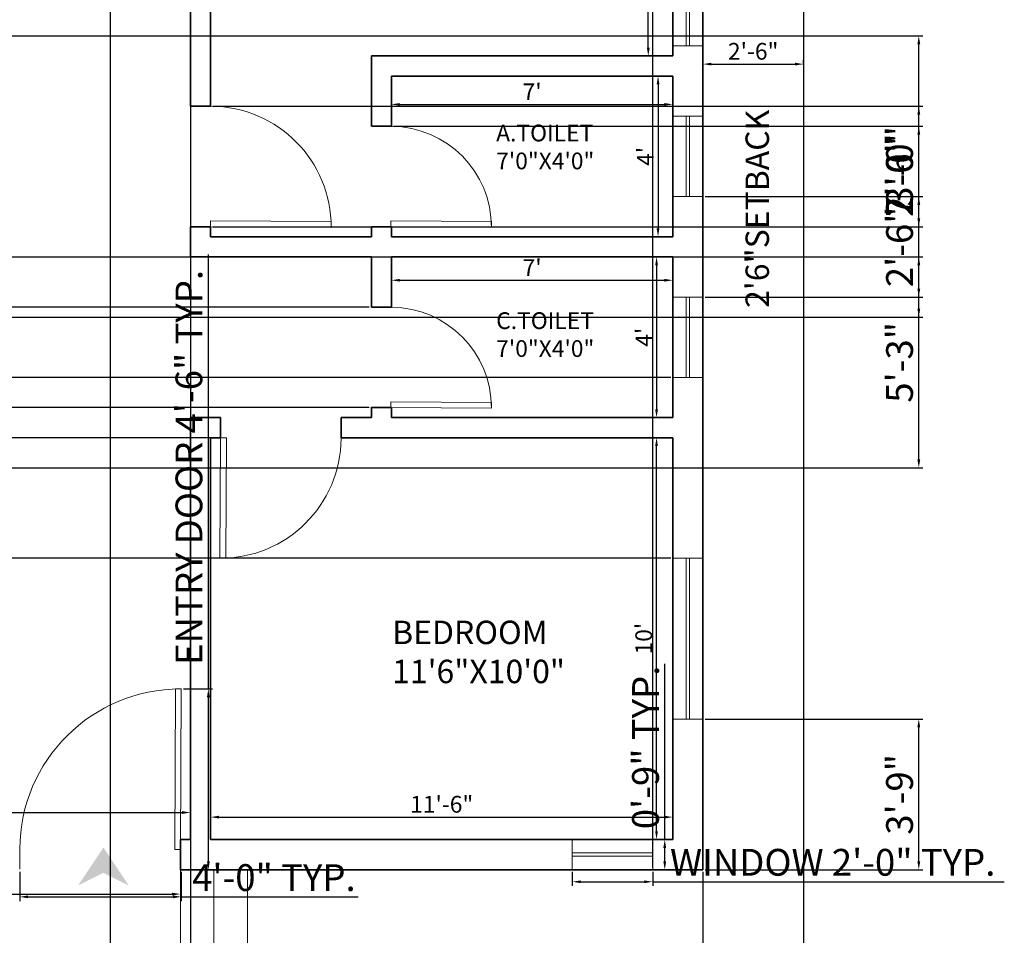
# Model space of a CAD drawing. Units: inches. Extents: x 3394 to 4794, y 965 to 1718.
# Tile 14 of 15: x 4500 to 4794, y 1179 to 1453. Entities that reach past the tile are written whole.
import ezdxf

# ---------------------------------------------------------------- set-up
doc = ezdxf.new("R2010")
doc.units = ezdxf.units.IN
for name, color, linetype, lineweight in [('A-ANNO-DIMS', 2, 'Continuous', 13), ('A-ANNO-PATT', 1, 'Continuous', 13), ('A-ANNO-TEXT', 7, 'Continuous', 18), ('A-AREA-IDEN', 7, 'Continuous', 18), ('A-DOOR', 4, 'Continuous', 18), ('A-FLOR-STRS', 7, 'Continuous', 18), ('A-GLAZ', 4, 'Continuous', 18), ('A-WALL', 7, 'Continuous', 35), ('C-PROP', 7, 'Continuous', 25)]:
    doc.layers.add(name, color=color, linetype=linetype, lineweight=lineweight)
doc.styles.get("Standard").update_dxf_attribs({"font": 'arial.ttf'})
doc.dimstyles.new('ISO-25', dxfattribs={"dimtxt": 8, "dimasz": 2.5, "dimexe": 1.25, "dimexo": 0.625, "dimtad": 1, "dimlunit": 3, "dimtxsty": 'Standard', "dimcen": 2.5, "dimadec": 0, "dimazin": 0, "dimtfac": 1, "dimtmove": 0, "dimatfit": 3, "dimfxl": 1, "dimarcsym": 0})

# ---------------------------------------------------------------- blocks, each defined once
blk = doc.blocks.new('*U5')
for p, q in [((0, 0), (0, -6)), ((30, 0), (30, -6))]:
    blk.add_line(p, q)
blk.add_lwpolyline([(0, 0), (0, 30), (1.75, 30), (1.75, 0)], close=True)
blk.add_arc((0, 0), 30, 0, 90)
blk = doc.blocks.new('*U11')
for p, q in [((0, 0), (0, -6)), ((36, 0), (36, -6))]:
    blk.add_line(p, q)
blk.add_lwpolyline([(0, 0), (0, 36), (1.75, 36), (1.75, 0)], close=True)
blk.add_arc((0, 0), 36, 0, 90)
blk = doc.blocks.new('*D36')
at = {"layer": 'A-ANNO-DIMS', "color": 0, "lineweight": -2, "transparency": 16777216}
for p, q in [((4419.27, 1198.06), (4419.27, 1190.15)), ((4548.27, 1198.06), (4548.27, 1190.15)), ((4421.77, 1191.4), (4545.77, 1191.4))]:
    blk.add_line(p, q, dxfattribs=at)
at = {"layer": 'A-ANNO-DIMS', "color": 0, "transparency": 16777216}
for points in [[(4421.77, 1191.81), (4421.77, 1190.98), (4419.27, 1191.4)], [(4545.77, 1191.81), (4545.77, 1190.98), (4548.27, 1191.4)]]:
    blk.add_solid(points, dxfattribs=at)
at = {"layer": 'Defpoints', "color": 0, "transparency": 16777216}
for p in [(4419.27, 1198.68), (4548.27, 1198.68), (4548.27, 1191.4)]:
    blk.add_point(p, dxfattribs=at)
at = {"layer": 'A-ANNO-DIMS', "color": 0, "transparency": 16777216, "insert": (4483.77, 1194.58), "char_height": 5, "attachment_point": 5}
blk.add_mtext('10\'-9"', dxfattribs=at)
blk = doc.blocks.new('*D38')
at = {"layer": 'A-ANNO-DIMS', "color": 0, "lineweight": -2, "transparency": 16777216}
for p, q in [((4704.27, 1439.09), (4704.27, 1440.48)), ((4706.77, 1439.23), (4731.77, 1439.23)), ((4734.27, 1439.09), (4734.27, 1440.48))]:
    blk.add_line(p, q, dxfattribs=at)
at = {"layer": 'A-ANNO-DIMS', "color": 0, "transparency": 16777216}
for points in [[(4706.77, 1439.65), (4706.77, 1438.82), (4704.27, 1439.23)], [(4731.77, 1439.65), (4731.77, 1438.82), (4734.27, 1439.23)]]:
    blk.add_solid(points, dxfattribs=at)
at = {"layer": 'Defpoints', "color": 0, "transparency": 16777216}
for p in [(4704.27, 1438.47), (4734.27, 1439.23), (4734.27, 1438.47)]:
    blk.add_point(p, dxfattribs=at)
at = {"layer": 'A-ANNO-DIMS', "color": 0, "transparency": 16777216, "insert": (4719.27, 1442.41), "char_height": 5, "attachment_point": 5}
blk.add_mtext('2\'-6"', dxfattribs=at)
blk = doc.blocks.new('*D41')
at = {"layer": 'A-ANNO-DIMS', "color": 0, "lineweight": -2, "transparency": 16777216}
for p, q in [((4350.27, 1208.31), (4350.27, 1217.01)), ((4352.77, 1215.76), (4548.77, 1215.76)), ((4551.27, 1208.31), (4551.27, 1217.01))]:
    blk.add_line(p, q, dxfattribs=at)
at = {"layer": 'A-ANNO-DIMS', "color": 0, "transparency": 16777216}
for points in [[(4352.77, 1216.17), (4352.77, 1215.34), (4350.27, 1215.76)], [(4548.77, 1216.17), (4548.77, 1215.34), (4551.27, 1215.76)]]:
    blk.add_solid(points, dxfattribs=at)
at = {"layer": 'Defpoints', "color": 0, "transparency": 16777216}
for p in [(4551.27, 1215.76), (4350.27, 1207.68), (4551.27, 1207.68)]:
    blk.add_point(p, dxfattribs=at)
at = {"layer": 'A-ANNO-DIMS', "color": 0, "transparency": 16777216, "insert": (4450.77, 1218.94), "char_height": 5, "attachment_point": 5}
blk.add_mtext('16\'-9"', dxfattribs=at)
blk = doc.blocks.new('*D42')
at = {"layer": 'A-ANNO-DIMS', "color": 0, "lineweight": -2, "transparency": 16777216}
for p, q in [((4557.27, 1208.31), (4557.27, 1215.64)), ((4559.77, 1214.39), (4692.77, 1214.39)), ((4695.27, 1208.31), (4695.27, 1215.64))]:
    blk.add_line(p, q, dxfattribs=at)
at = {"layer": 'A-ANNO-DIMS', "color": 0, "transparency": 16777216}
for points in [[(4559.77, 1214.8), (4559.77, 1213.97), (4557.27, 1214.39)], [(4692.77, 1214.8), (4692.77, 1213.97), (4695.27, 1214.39)]]:
    blk.add_solid(points, dxfattribs=at)
at = {"layer": 'Defpoints', "color": 0, "transparency": 16777216}
for p in [(4695.27, 1214.39), (4557.27, 1207.68), (4695.27, 1207.68)]:
    blk.add_point(p, dxfattribs=at)
at = {"layer": 'A-ANNO-DIMS', "color": 0, "transparency": 16777216, "insert": (4626.27, 1217.57), "char_height": 5, "attachment_point": 5}
blk.add_mtext('11\'-6"', dxfattribs=at)
blk = doc.blocks.new('*D43')
at = {"layer": 'A-ANNO-DIMS', "color": 0, "lineweight": -2, "transparency": 16777216}
for p, q in [((4694.65, 1327.68), (4689.17, 1327.68)), ((4690.42, 1210.18), (4690.42, 1325.18)), ((4694.65, 1207.68), (4689.17, 1207.68))]:
    blk.add_line(p, q, dxfattribs=at)
at = {"layer": 'A-ANNO-DIMS', "color": 0, "transparency": 16777216}
for points in [[(4690, 1325.18), (4690.83, 1325.18), (4690.42, 1327.68)], [(4690, 1210.18), (4690.83, 1210.18), (4690.42, 1207.68)]]:
    blk.add_solid(points, dxfattribs=at)
at = {"layer": 'Defpoints', "color": 0, "transparency": 16777216}
for p in [(4690.42, 1327.68), (4695.27, 1327.68), (4695.27, 1207.68)]:
    blk.add_point(p, dxfattribs=at)
at = {"layer": 'A-ANNO-DIMS', "color": 0, "transparency": 16777216, "insert": (4687.24, 1267.68), "char_height": 5, "attachment_point": 5, "rotation": 90}
blk.add_mtext("10'", dxfattribs=at)
blk = doc.blocks.new('*D44')
at = {"layer": 'A-ANNO-DIMS', "color": 0, "lineweight": -2, "transparency": 16777216}
for p, q in [((4611.27, 1381.06), (4611.27, 1373.45)), ((4695.27, 1381.06), (4695.27, 1373.45)), ((4613.77, 1374.7), (4692.77, 1374.7))]:
    blk.add_line(p, q, dxfattribs=at)
at = {"layer": 'A-ANNO-DIMS', "color": 0, "transparency": 16777216}
for points in [[(4613.77, 1375.11), (4613.77, 1374.28), (4611.27, 1374.7)], [(4692.77, 1375.11), (4692.77, 1374.28), (4695.27, 1374.7)]]:
    blk.add_solid(points, dxfattribs=at)
at = {"layer": 'Defpoints', "color": 0, "transparency": 16777216}
for p in [(4611.27, 1381.68), (4695.27, 1381.68), (4695.27, 1374.7)]:
    blk.add_point(p, dxfattribs=at)
at = {"layer": 'A-ANNO-DIMS', "color": 0, "transparency": 16777216, "insert": (4653.27, 1377.82), "char_height": 5, "attachment_point": 5}
blk.add_mtext("7'", dxfattribs=at)
blk = doc.blocks.new('*D45')
at = {"layer": 'A-ANNO-DIMS', "color": 0, "lineweight": -2, "transparency": 16777216}
for p, q in [((4694.65, 1381.68), (4689.18, 1381.68)), ((4690.43, 1379.18), (4690.43, 1336.18)), ((4694.65, 1333.68), (4689.18, 1333.68))]:
    blk.add_line(p, q, dxfattribs=at)
at = {"layer": 'A-ANNO-DIMS', "color": 0, "transparency": 16777216}
for points in [[(4690.01, 1379.18), (4690.84, 1379.18), (4690.43, 1381.68)], [(4690.01, 1336.18), (4690.84, 1336.18), (4690.43, 1333.68)]]:
    blk.add_solid(points, dxfattribs=at)
at = {"layer": 'Defpoints', "color": 0, "transparency": 16777216}
for p in [(4695.27, 1381.68), (4690.43, 1333.68), (4695.27, 1333.68)]:
    blk.add_point(p, dxfattribs=at)
at = {"layer": 'A-ANNO-DIMS', "color": 0, "transparency": 16777216, "insert": (4687.3, 1357.68), "char_height": 5, "attachment_point": 5, "rotation": 90}
blk.add_mtext("4'", dxfattribs=at)
blk = doc.blocks.new('*D46')
at = {"layer": 'A-ANNO-DIMS', "color": 0, "lineweight": -2, "transparency": 16777216}
for p, q in [((4694.65, 1435.68), (4689.62, 1435.68)), ((4690.87, 1433.18), (4690.87, 1390.18)), ((4694.65, 1387.68), (4689.62, 1387.68))]:
    blk.add_line(p, q, dxfattribs=at)
at = {"layer": 'A-ANNO-DIMS', "color": 0, "transparency": 16777216}
for points in [[(4690.45, 1433.18), (4691.28, 1433.18), (4690.87, 1435.68)], [(4690.45, 1390.18), (4691.28, 1390.18), (4690.87, 1387.68)]]:
    blk.add_solid(points, dxfattribs=at)
at = {"layer": 'Defpoints', "color": 0, "transparency": 16777216}
for p in [(4695.27, 1435.68), (4690.87, 1387.68), (4695.27, 1387.68)]:
    blk.add_point(p, dxfattribs=at)
at = {"layer": 'A-ANNO-DIMS', "color": 0, "transparency": 16777216, "insert": (4687.74, 1411.68), "char_height": 5, "attachment_point": 5, "rotation": 90}
blk.add_mtext("4'", dxfattribs=at)
blk = doc.blocks.new('*D47')
at = {"layer": 'A-ANNO-DIMS', "color": 0, "lineweight": -2, "transparency": 16777216}
for p, q in [((4611.27, 1435.06), (4611.27, 1425.96)), ((4695.27, 1435.06), (4695.27, 1425.96)), ((4613.77, 1427.21), (4692.77, 1427.21))]:
    blk.add_line(p, q, dxfattribs=at)
at = {"layer": 'A-ANNO-DIMS', "color": 0, "transparency": 16777216}
for points in [[(4613.77, 1427.62), (4613.77, 1426.79), (4611.27, 1427.21)], [(4692.77, 1427.62), (4692.77, 1426.79), (4695.27, 1427.21)]]:
    blk.add_solid(points, dxfattribs=at)
at = {"layer": 'Defpoints', "color": 0, "transparency": 16777216}
for p in [(4611.27, 1435.68), (4695.27, 1435.68), (4695.27, 1427.21)]:
    blk.add_point(p, dxfattribs=at)
at = {"layer": 'A-ANNO-DIMS', "color": 0, "transparency": 16777216, "insert": (4653.27, 1430.33), "char_height": 5, "attachment_point": 5}
blk.add_mtext("7'", dxfattribs=at)
blk = doc.blocks.new('*D48')
at = {"layer": 'A-ANNO-DIMS', "color": 0, "lineweight": -2, "transparency": 16777216}
for p, q in [((4694.65, 1573.68), (4686.7, 1573.68)), ((4687.95, 1444.18), (4687.95, 1571.18)), ((4694.65, 1441.68), (4686.7, 1441.68))]:
    blk.add_line(p, q, dxfattribs=at)
at = {"layer": 'A-ANNO-DIMS', "color": 0, "transparency": 16777216}
for points in [[(4687.53, 1571.18), (4688.37, 1571.18), (4687.95, 1573.68)], [(4687.53, 1444.18), (4688.37, 1444.18), (4687.95, 1441.68)]]:
    blk.add_solid(points, dxfattribs=at)
at = {"layer": 'Defpoints', "color": 0, "transparency": 16777216}
for p in [(4687.95, 1573.68), (4695.27, 1573.68), (4695.27, 1441.68)]:
    blk.add_point(p, dxfattribs=at)
at = {"layer": 'A-ANNO-DIMS', "color": 0, "transparency": 16777216, "insert": (4684.81, 1507.68), "char_height": 5, "attachment_point": 5, "rotation": 90}
blk.add_mtext("11'", dxfattribs=at)
blk = doc.blocks.new('WIN-48IN')
for p, q in [((9, 48), (0, 48)), ((4, 0), (4, 48)), ((5, 0), (5, 48)), ((9, 0), (0, 0))]:
    blk.add_line(p, q)
blk = doc.blocks.new('WIN-24IN')
for p, q in [((0, 9), (0, 0)), ((24, 9), (24, 0)), ((0, 5), (24, 5)), ((0, 4), (24, 4))]:
    blk.add_line(p, q)
blk = doc.blocks.new('DOOR-ENTRY-48IN')
for p, q in [((0.03, 6.2), (0, 0.2)), ((48.03, 6), (48, 0))]:
    blk.add_line(p, q)
blk.add_lwpolyline([(48.03, 6), (48.24, 54), (46.49, 54.01), (46.28, 6.01)], close=True)
blk.add_arc((48.03, 6), 48, 90, 179.759)
blk = doc.blocks.new('STAIR-SITOUT-3STEP')
for p, q in [((129, 68), (129, 20)), ((139, 68), (139, 10)), ((149, 68), (149, 0)), ((0, 20), (129, 20)), ((0, 10), (139, 10)), ((0, 0), (149, 0))]:
    blk.add_line(p, q)
blk = doc.blocks.new('*D64')
at = {"layer": 'A-ANNO-DIMS', "color": 0, "lineweight": -2, "transparency": 16777216}
for p, q in [((4665.27, 1198.06), (4665.27, 1193.83)), ((4689.27, 1198.06), (4689.27, 1193.83)), ((4667.77, 1195.08), (4686.77, 1195.08)), ((4689.27, 1195.08), (4794.25, 1195.08))]:
    blk.add_line(p, q, dxfattribs=at)
at = {"layer": 'A-ANNO-DIMS', "color": 0, "transparency": 16777216}
for points in [[(4667.77, 1195.5), (4667.77, 1194.67), (4665.27, 1195.08)], [(4686.77, 1195.5), (4686.77, 1194.67), (4689.27, 1195.08)]]:
    blk.add_solid(points, dxfattribs=at)
at = {"layer": 'Defpoints', "color": 0, "transparency": 16777216}
for p in [(4665.27, 1198.68), (4689.27, 1198.68), (4689.27, 1195.08)]:
    blk.add_point(p, dxfattribs=at)
at = {"layer": 'A-ANNO-DIMS', "color": 0, "transparency": 16777216, "insert": (4743.01, 1199.85), "char_height": 8, "attachment_point": 5}
blk.add_mtext('WINDOW 2\'-0" TYP.', dxfattribs=at)
blk = doc.blocks.new('*D65')
at = {"layer": 'A-ANNO-DIMS', "color": 0, "lineweight": -2, "transparency": 16777216}
for p, q in [((4692.87, 1207.68), (4692.87, 1260.2)), ((4689.9, 1207.68), (4694.12, 1207.68)), ((4692.87, 1201.18), (4692.87, 1205.18)), ((4689.9, 1198.68), (4694.12, 1198.68))]:
    blk.add_line(p, q, dxfattribs=at)
at = {"layer": 'A-ANNO-DIMS', "color": 0, "transparency": 16777216}
for points in [[(4692.45, 1205.18), (4693.29, 1205.18), (4692.87, 1207.68)], [(4692.45, 1201.18), (4693.29, 1201.18), (4692.87, 1198.68)]]:
    blk.add_solid(points, dxfattribs=at)
at = {"layer": 'Defpoints', "color": 0, "transparency": 16777216}
for p in [(4689.27, 1207.68), (4692.87, 1207.68), (4689.27, 1198.68)]:
    blk.add_point(p, dxfattribs=at)
at = {"layer": 'A-ANNO-DIMS', "color": 0, "transparency": 16777216, "insert": (4688.16, 1235.19), "char_height": 8, "attachment_point": 5, "rotation": 90}
blk.add_mtext('0\'-9" TYP.', dxfattribs=at)
blk = doc.blocks.new('*D68')
at = {"layer": 'A-ANNO-DIMS', "color": 0, "lineweight": -2, "transparency": 16777216}
for p, q in [((4556.61, 1252.69), (4556.61, 1382.4)), ((4549.13, 1252.69), (4557.86, 1252.69)), ((4556.61, 1201.18), (4556.61, 1250.19)), ((4549.13, 1198.68), (4557.86, 1198.68))]:
    blk.add_line(p, q, dxfattribs=at)
at = {"layer": 'A-ANNO-DIMS', "color": 0, "transparency": 16777216}
for points in [[(4556.19, 1250.19), (4557.02, 1250.19), (4556.61, 1252.69)], [(4556.19, 1201.18), (4557.02, 1201.18), (4556.61, 1198.68)]]:
    blk.add_solid(points, dxfattribs=at)
at = {"layer": 'Defpoints', "color": 0, "transparency": 16777216}
for p in [(4548.51, 1252.69), (4556.61, 1252.69), (4548.51, 1198.68)]:
    blk.add_point(p, dxfattribs=at)
at = {"layer": 'A-ANNO-DIMS', "color": 0, "transparency": 16777216, "insert": (4551.84, 1318.8), "char_height": 8, "attachment_point": 5, "rotation": 90}
blk.add_mtext('ENTRY DOOR 4\'-6" TYP.', dxfattribs=at)
blk = doc.blocks.new('*D69')
at = {"layer": 'A-ANNO-DIMS', "color": 0, "lineweight": -2, "transparency": 16777216}
for p, q in [((4500.27, 1198.06), (4500.27, 1189.33)), ((4548.51, 1198.06), (4548.51, 1189.33)), ((4502.77, 1190.58), (4546.01, 1190.58)), ((4548.51, 1190.58), (4601.34, 1190.58))]:
    blk.add_line(p, q, dxfattribs=at)
at = {"layer": 'A-ANNO-DIMS', "color": 0, "transparency": 16777216}
for points in [[(4502.77, 1191), (4502.77, 1190.16), (4500.27, 1190.58)], [(4546.01, 1191), (4546.01, 1190.16), (4548.51, 1190.58)]]:
    blk.add_solid(points, dxfattribs=at)
at = {"layer": 'Defpoints', "color": 0, "transparency": 16777216}
for p in [(4500.27, 1198.68), (4548.51, 1198.68), (4548.51, 1190.58)]:
    blk.add_point(p, dxfattribs=at)
at = {"layer": 'A-ANNO-DIMS', "color": 0, "transparency": 16777216, "insert": (4576.17, 1195.29), "char_height": 8, "attachment_point": 5}
blk.add_mtext('4\'-0" TYP.', dxfattribs=at)
blk = doc.blocks.new('*D106')
at = {"layer": 'A-ANNO-DIMS', "color": 0, "lineweight": -2, "transparency": 16777216}
for p, q in [((4704.27, 1198.06), (4704.27, 987.36)), ((4341.27, 1117.06), (4341.27, 987.36)), ((4343.77, 988.61), (4701.77, 988.61))]:
    blk.add_line(p, q, dxfattribs=at)
at = {"layer": 'A-ANNO-DIMS', "color": 0, "transparency": 16777216}
for points in [[(4343.77, 989.03), (4343.77, 988.2), (4341.27, 988.61)], [(4701.77, 989.03), (4701.77, 988.2), (4704.27, 988.61)]]:
    blk.add_solid(points, dxfattribs=at)
at = {"layer": 'Defpoints', "color": 0, "transparency": 16777216}
for p in [(4704.27, 1198.68), (4341.27, 1117.68), (4704.27, 988.61)]:
    blk.add_point(p, dxfattribs=at)
at = {"layer": 'A-ANNO-DIMS', "color": 0, "transparency": 16777216, "insert": (4522.77, 993.32), "char_height": 8, "attachment_point": 5}
blk.add_mtext('30\'-3"', dxfattribs=at)
blk = doc.blocks.new('*D109')
at = {"layer": 'A-ANNO-DIMS', "color": 0, "lineweight": -2, "transparency": 16777216}
for p, q in [((4456.9, 1447.68), (4769.97, 1447.68)), ((4768.72, 1366.18), (4768.72, 1445.18)), ((4456.9, 1363.68), (4769.97, 1363.68))]:
    blk.add_line(p, q, dxfattribs=at)
at = {"layer": 'A-ANNO-DIMS', "color": 0, "transparency": 16777216}
for points in [[(4768.3, 1445.18), (4769.14, 1445.18), (4768.72, 1447.68)], [(4768.3, 1366.18), (4769.14, 1366.18), (4768.72, 1363.68)]]:
    blk.add_solid(points, dxfattribs=at)
at = {"layer": 'Defpoints', "color": 0, "transparency": 16777216}
for p in [(4456.27, 1447.68), (4768.72, 1447.68), (4456.27, 1363.68)]:
    blk.add_point(p, dxfattribs=at)
at = {"layer": 'A-ANNO-DIMS', "color": 0, "transparency": 16777216, "insert": (4764.01, 1405.68), "char_height": 8, "attachment_point": 5, "rotation": 90}
blk.add_mtext('7\'-0"', dxfattribs=at)
blk = doc.blocks.new('*D110')
at = {"layer": 'A-ANNO-DIMS', "color": 0, "lineweight": -2, "transparency": 16777216}
for p, q in [((4557.9, 1426.68), (4769.97, 1426.68)), ((4768.72, 1393.18), (4768.72, 1424.18)), ((4557.9, 1390.68), (4769.97, 1390.68))]:
    blk.add_line(p, q, dxfattribs=at)
at = {"layer": 'A-ANNO-DIMS', "color": 0, "transparency": 16777216}
for points in [[(4768.3, 1424.18), (4769.14, 1424.18), (4768.72, 1426.68)], [(4768.3, 1393.18), (4769.14, 1393.18), (4768.72, 1390.68)]]:
    blk.add_solid(points, dxfattribs=at)
at = {"layer": 'Defpoints', "color": 0, "transparency": 16777216}
for p in [(4557.27, 1426.68), (4768.72, 1426.68), (4557.27, 1390.68)]:
    blk.add_point(p, dxfattribs=at)
at = {"layer": 'A-ANNO-DIMS', "color": 0, "transparency": 16777216, "insert": (4764.01, 1408.68), "char_height": 8, "attachment_point": 5, "rotation": 90}
blk.add_mtext('3\'-0"', dxfattribs=at)
blk = doc.blocks.new('*D111')
at = {"layer": 'A-ANNO-DIMS', "color": 0, "lineweight": -2, "transparency": 16777216}
for p, q in [((4611.9, 1420.68), (4769.97, 1420.68)), ((4768.72, 1393.18), (4768.72, 1418.18)), ((4611.9, 1390.68), (4769.97, 1390.68))]:
    blk.add_line(p, q, dxfattribs=at)
at = {"layer": 'A-ANNO-DIMS', "color": 0, "transparency": 16777216}
for points in [[(4768.3, 1418.18), (4769.14, 1418.18), (4768.72, 1420.68)], [(4768.3, 1393.18), (4769.14, 1393.18), (4768.72, 1390.68)]]:
    blk.add_solid(points, dxfattribs=at)
at = {"layer": 'Defpoints', "color": 0, "transparency": 16777216}
for p in [(4611.27, 1420.68), (4768.72, 1420.68), (4611.27, 1390.68)]:
    blk.add_point(p, dxfattribs=at)
at = {"layer": 'A-ANNO-DIMS', "color": 0, "transparency": 16777216, "insert": (4764.01, 1405.68), "char_height": 8, "attachment_point": 5, "rotation": 90}
blk.add_mtext('2\'-6"', dxfattribs=at)
blk = doc.blocks.new('*D112')
at = {"layer": 'A-ANNO-DIMS', "color": 0, "lineweight": -2, "transparency": 16777216}
for p, q in [((4559.65, 1327.68), (4185.57, 1327.68)), ((4186.82, 1294.18), (4186.82, 1325.18)), ((4559.41, 1291.68), (4185.57, 1291.68))]:
    blk.add_line(p, q, dxfattribs=at)
at = {"layer": 'A-ANNO-DIMS', "color": 0, "transparency": 16777216}
for points in [[(4186.4, 1325.18), (4187.24, 1325.18), (4186.82, 1327.68)], [(4186.4, 1294.18), (4187.24, 1294.18), (4186.82, 1291.68)]]:
    blk.add_solid(points, dxfattribs=at)
at = {"layer": 'Defpoints', "color": 0, "transparency": 16777216}
for p in [(4186.82, 1327.68), (4560.27, 1327.68), (4560.03, 1291.68)]:
    blk.add_point(p, dxfattribs=at)
at = {"layer": 'A-ANNO-DIMS', "color": 0, "transparency": 16777216, "insert": (4182.11, 1309.68), "char_height": 8, "attachment_point": 5, "rotation": 90}
blk.add_mtext('3\'-0"', dxfattribs=at)
blk = doc.blocks.new('*D113')
at = {"layer": 'A-ANNO-DIMS', "color": 0, "lineweight": -2, "transparency": 16777216}
for p, q in [((4604.65, 1366.68), (4185.57, 1366.68)), ((4186.82, 1339.18), (4186.82, 1364.18)), ((4604.65, 1336.68), (4185.57, 1336.68))]:
    blk.add_line(p, q, dxfattribs=at)
at = {"layer": 'A-ANNO-DIMS', "color": 0, "transparency": 16777216}
for points in [[(4186.4, 1364.18), (4187.24, 1364.18), (4186.82, 1366.68)], [(4186.4, 1339.18), (4187.24, 1339.18), (4186.82, 1336.68)]]:
    blk.add_solid(points, dxfattribs=at)
at = {"layer": 'Defpoints', "color": 0, "transparency": 16777216}
for p in [(4186.82, 1366.68), (4605.27, 1366.68), (4605.27, 1336.68)]:
    blk.add_point(p, dxfattribs=at)
at = {"layer": 'A-ANNO-DIMS', "color": 0, "transparency": 16777216, "insert": (4182.11, 1351.68), "char_height": 8, "attachment_point": 5, "rotation": 90}
blk.add_mtext('2\'-6"', dxfattribs=at)
blk = doc.blocks.new('*D116')
at = {"layer": 'A-ANNO-DIMS', "color": 0, "lineweight": -2, "transparency": 16777216}
for p, q in [((4350.9, 1381.68), (4769.97, 1381.68)), ((4768.72, 1321.18), (4768.72, 1379.18)), ((4350.9, 1318.68), (4769.97, 1318.68))]:
    blk.add_line(p, q, dxfattribs=at)
at = {"layer": 'A-ANNO-DIMS', "color": 0, "transparency": 16777216}
for points in [[(4768.3, 1379.18), (4769.14, 1379.18), (4768.72, 1381.68)], [(4768.3, 1321.18), (4769.14, 1321.18), (4768.72, 1318.68)]]:
    blk.add_solid(points, dxfattribs=at)
at = {"layer": 'Defpoints', "color": 0, "transparency": 16777216}
for p in [(4350.27, 1381.68), (4768.72, 1381.68), (4350.27, 1318.68)]:
    blk.add_point(p, dxfattribs=at)
at = {"layer": 'A-ANNO-DIMS', "color": 0, "transparency": 16777216, "insert": (4764.01, 1350.18), "char_height": 8, "attachment_point": 5, "rotation": 90}
blk.add_mtext('5\'-3"', dxfattribs=at)
blk = doc.blocks.new('*D118')
at = {"layer": 'A-ANNO-DIMS', "color": 0, "lineweight": -2, "transparency": 16777216}
for p, q in [((4704.9, 1243.68), (4769.97, 1243.68)), ((4768.72, 1201.18), (4768.72, 1241.18)), ((4704.9, 1198.68), (4769.97, 1198.68))]:
    blk.add_line(p, q, dxfattribs=at)
at = {"layer": 'A-ANNO-DIMS', "color": 0, "transparency": 16777216}
for points in [[(4768.3, 1241.18), (4769.14, 1241.18), (4768.72, 1243.68)], [(4768.3, 1201.18), (4769.14, 1201.18), (4768.72, 1198.68)]]:
    blk.add_solid(points, dxfattribs=at)
at = {"layer": 'Defpoints', "color": 0, "transparency": 16777216}
for p in [(4704.27, 1243.68), (4768.72, 1243.68), (4704.27, 1198.68)]:
    blk.add_point(p, dxfattribs=at)
at = {"layer": 'A-ANNO-DIMS', "color": 0, "transparency": 16777216, "insert": (4764.01, 1221.18), "char_height": 8, "attachment_point": 5, "rotation": 90}
blk.add_mtext('3\'-9"', dxfattribs=at)
blk = doc.blocks.new('*D119')
at = {"layer": 'A-ANNO-DIMS', "color": 0, "lineweight": -2, "transparency": 16777216}
for p, q in [((4694.65, 1345.68), (4185.57, 1345.68)), ((4186.82, 1294.18), (4186.82, 1343.18)), ((4694.65, 1291.68), (4185.57, 1291.68))]:
    blk.add_line(p, q, dxfattribs=at)
at = {"layer": 'A-ANNO-DIMS', "color": 0, "transparency": 16777216}
for points in [[(4186.4, 1343.18), (4187.24, 1343.18), (4186.82, 1345.68)], [(4186.4, 1294.18), (4187.24, 1294.18), (4186.82, 1291.68)]]:
    blk.add_solid(points, dxfattribs=at)
at = {"layer": 'Defpoints', "color": 0, "transparency": 16777216}
for p in [(4186.82, 1345.68), (4695.27, 1345.68), (4695.27, 1291.68)]:
    blk.add_point(p, dxfattribs=at)
at = {"layer": 'A-ANNO-DIMS', "color": 0, "transparency": 16777216, "insert": (4182.11, 1318.68), "char_height": 8, "attachment_point": 5, "rotation": 90}
blk.add_mtext('4\'-6"', dxfattribs=at)
blk = doc.blocks.new('*D120')
at = {"layer": 'A-ANNO-DIMS', "color": 0, "lineweight": -2, "transparency": 16777216}
for p, q in [((4704.9, 1399.68), (4769.97, 1399.68)), ((4768.72, 1372.18), (4768.72, 1397.18)), ((4704.9, 1369.68), (4769.97, 1369.68))]:
    blk.add_line(p, q, dxfattribs=at)
at = {"layer": 'A-ANNO-DIMS', "color": 0, "transparency": 16777216}
for points in [[(4768.3, 1397.18), (4769.14, 1397.18), (4768.72, 1399.68)], [(4768.3, 1372.18), (4769.14, 1372.18), (4768.72, 1369.68)]]:
    blk.add_solid(points, dxfattribs=at)
at = {"layer": 'Defpoints', "color": 0, "transparency": 16777216}
for p in [(4704.27, 1399.68), (4768.72, 1399.68), (4704.27, 1369.68)]:
    blk.add_point(p, dxfattribs=at)
at = {"layer": 'A-ANNO-DIMS', "color": 0, "transparency": 16777216, "insert": (4764.01, 1384.68), "char_height": 8, "attachment_point": 5, "rotation": 90}
blk.add_mtext('2\'-6"', dxfattribs=at)
blk = doc.blocks.new('*D122')
at = {"layer": 'A-ANNO-DIMS', "color": 0, "lineweight": -2, "transparency": 16777216}
for p, q in [((4689.27, 1199.31), (4689.27, 1702.38)), ((4704.27, 1199.31), (4704.27, 1702.38)), ((4691.77, 1701.13), (4701.77, 1701.13)), ((4704.27, 1701.13), (4728.53, 1701.13))]:
    blk.add_line(p, q, dxfattribs=at)
at = {"layer": 'A-ANNO-DIMS', "color": 0, "transparency": 16777216}
for points in [[(4691.77, 1701.55), (4691.77, 1700.72), (4689.27, 1701.13)], [(4701.77, 1701.55), (4701.77, 1700.72), (4704.27, 1701.13)]]:
    blk.add_solid(points, dxfattribs=at)
at = {"layer": 'Defpoints', "color": 0, "transparency": 16777216}
for p in [(4704.27, 1701.13), (4689.27, 1198.68), (4704.27, 1198.68)]:
    blk.add_point(p, dxfattribs=at)
at = {"layer": 'A-ANNO-DIMS', "color": 0, "transparency": 16777216, "insert": (4717.65, 1705.84), "char_height": 8, "attachment_point": 5}
blk.add_mtext('1\'-3"', dxfattribs=at)
blk = doc.blocks.new('*D128')
at = {"layer": 'A-ANNO-DIMS', "color": 0, "lineweight": -2, "transparency": 16777216}
for p, q in [((4527.27, 1573.06), (4527.27, 987.36)), ((4551.27, 1573.06), (4551.27, 987.36)), ((4529.77, 988.61), (4548.77, 988.61))]:
    blk.add_line(p, q, dxfattribs=at)
at = {"layer": 'A-ANNO-DIMS', "color": 0, "transparency": 16777216}
for points in [[(4529.77, 989.03), (4529.77, 988.2), (4527.27, 988.61)], [(4548.77, 989.03), (4548.77, 988.2), (4551.27, 988.61)]]:
    blk.add_solid(points, dxfattribs=at)
at = {"layer": 'Defpoints', "color": 0, "transparency": 16777216}
for p in [(4527.27, 1573.68), (4551.27, 1573.68), (4551.27, 988.61)]:
    blk.add_point(p, dxfattribs=at)
at = {"layer": 'A-ANNO-DIMS', "color": 0, "transparency": 16777216, "insert": (4539.27, 993.32), "char_height": 8, "attachment_point": 5}
blk.add_mtext('2\'-0"', dxfattribs=at)

msp = doc.modelspace()

# ---------------------------------------------------------------- hatches: boundary and pattern name
at = {"layer": 'A-ANNO-PATT'}
h = msp.add_hatch(color=256, dxfattribs=at)
h.dxf.hatch_style = 1
h.paths.add_polyline_path([(4525.267, 1205.307), (4517.716, 1193.982), (4525.267, 1197.757), (4532.817, 1193.982)])

# ---------------------------------------------------------------- linework, layer by layer
at = {"layer": 'A-WALL'}
for p, q in [((4557.27, 1582.682), (4557.27, 1426.682)), ((4704.27, 1582.682), (4704.27, 1198.682)), ((4551.27, 1573.682), (4551.27, 1426.682)), ((4695.27, 1573.682), (4695.27, 1441.682)), ((4605.27, 1441.682), (4695.27, 1441.682)), ((4605.27, 1441.682), (4605.27, 1420.682)), ((4611.27, 1435.682), (4695.27, 1435.682)), ((4611.27, 1435.682), (4611.27, 1420.682)), ((4695.27, 1435.682), (4695.27, 1387.682)), ((4551.27, 1426.682), (4557.27, 1426.682)), ((4605.27, 1420.682), (4611.27, 1420.682)), ((4551.27, 1390.682), (4557.27, 1390.682)), ((4551.27, 1390.682), (4551.27, 1381.682)), ((4557.27, 1390.682), (4557.27, 1387.682)), ((4605.27, 1390.682), (4611.27, 1390.682)), ((4605.27, 1390.682), (4605.27, 1387.682)), ((4611.27, 1390.682), (4611.27, 1387.682)), ((4557.27, 1387.682), (4605.27, 1387.682)), ((4611.27, 1387.682), (4695.27, 1387.682)), ((4551.27, 1381.682), (4605.27, 1381.682)), ((4605.27, 1381.682), (4605.27, 1366.682)), ((4611.27, 1381.682), (4695.27, 1381.682)), ((4611.27, 1381.682), (4611.27, 1366.682)), ((4695.27, 1381.682), (4695.27, 1333.682)), ((4605.27, 1366.682), (4611.27, 1366.682)), ((4605.27, 1336.682), (4605.27, 1333.682)), ((4605.27, 1336.682), (4611.27, 1336.682)), ((4611.27, 1336.682), (4611.27, 1333.682)), ((4551.27, 1333.682), (4560.27, 1333.682)), ((4551.27, 1333.682), (4551.27, 1207.682)), ((4560.27, 1333.682), (4560.27, 1327.682)), ((4596.27, 1333.682), (4605.27, 1333.682)), ((4596.27, 1333.682), (4596.27, 1327.682)), ((4611.27, 1333.682), (4695.27, 1333.682)), ((4557.27, 1327.682), (4560.27, 1327.682)), ((4557.27, 1327.682), (4557.27, 1207.682)), ((4596.27, 1327.682), (4695.27, 1327.682)), ((4695.27, 1327.682), (4695.27, 1207.682)), ((4548.27, 1207.682), (4551.27, 1207.682)), ((4548.27, 1207.682), (4548.27, 1198.682)), ((4557.27, 1207.682), (4695.27, 1207.682)), ((4548.27, 1198.682), (4704.27, 1198.682))]:
    msp.add_line(p, q, dxfattribs=at)
at = {"layer": 'C-PROP'}
msp.add_line((4734.27, 1666.682), (4734.27, 1057.682), dxfattribs=at)

# ---------------------------------------------------------------- block references
at = {"layer": 'A-DOOR', "xscale": -1}
for name, p, rotation in [('*U11', (4557.27, 1390.649), 269.6786649249896), ('*U5', (4611.102, 1390.649), 269.6786649249897), ('*U5', (4611.102, 1336.649), 269.6786649249897), ('*U11', (4560.237, 1327.682), 179.6786649249896)]:
    msp.add_blockref(name, p, dxfattribs=dict(at, rotation=rotation))
at = {"layer": 'A-DOOR'}
msp.add_blockref('DOOR-ENTRY-48IN', (4500.271, 1198.682), dxfattribs=at)
at = {"layer": 'A-FLOR-STRS'}
msp.add_blockref('STAIR-SITOUT-3STEP', (4419.271, 1130.682), dxfattribs=at)
at = {"layer": 'A-GLAZ'}
for name, p in [('WIN-48IN', (4695.271, 1444.682)), ('WIN-48IN', (4695.271, 1243.682)), ('WIN-24IN', (4665.271, 1198.682))]:
    msp.add_blockref(name, p, dxfattribs=at)
for p, rotation in [((4695.27, 1423.682), 270.0000000000056), ((4704.271, 1345.683), 90.00000000000142)]:
    msp.add_blockref('WIN-24IN', p, dxfattribs=dict(at, rotation=rotation))

# ---------------------------------------------------------------- texts
at = {"layer": 'A-ANNO-TEXT', "insert": (4716.99, 1366.45), "char_height": 7, "attachment_point": 1, "rotation": 90}
msp.add_mtext_dynamic_manual_height_columns('{\\fTimes New Roman|b0|i0|c0|p18;2\'6"SETBACK}', width=61.05572, gutter_width=12.5, heights=[0], dxfattribs=at)
at = {"layer": 'A-AREA-IDEN', "attachment_point": 1}
for s, insert, char_height in [('{\\fTimes New Roman|b0|i0|c0|p18;A.TOILET\\P7\'0"X4\'0"}', (4642.534, 1421.162), 5), ('{\\fTimes New Roman|b0|i0|c0|p18;C.TOILET\\P7\'0"X4\'0"}', (4642.534, 1365.131), 5), ('{\\fTimes New Roman|b0|i0|c0|p18;BEDROOM\\P11\'6"X10\'0"}', (4611.465, 1273.048), 7)]:
    msp.add_mtext_dynamic_manual_height_columns(s, width=61.05572, gutter_width=12.5, heights=[0], dxfattribs=dict(at, insert=insert, char_height=char_height))

# ---------------------------------------------------------------- dimensions: what is measured, and where the dimension line sits
at = {"layer": 'A-ANNO-DIMS'}
for base, p1, p2, override, picture, middle in [((4704.27, 1701.132), (4689.27, 1198.682), (4704.27, 1198.682), {"dimdec": 1, "dimlfac": 1, "dimrnd": 0, "dimzin": 1, "dimdsep": 46, "dimlunit": 4, "dimfrac": 2}, '*D122', (4717.652, 1705.845)), ((4551.27, 988.612), (4527.27, 1573.682), (4551.27, 1573.682), {"dimdec": 1, "dimlfac": 1, "dimrnd": 0, "dimzin": 1, "dimdsep": 46, "dimlunit": 4, "dimfrac": 2}, '*D128', (4539.27, 993.322)), ((4734.27, 1439.233), (4704.27, 1438.468), (4734.27, 1438.468), {"dimtxt": 5, "dimclrd": 0, "dimclre": 0, "dimclrt": 0}, '*D38', (4719.27, 1442.411)), ((4695.27, 1427.207), (4611.27, 1435.682), (4695.27, 1435.682), {"dimtxt": 5, "dimclrd": 0, "dimclre": 0, "dimclrt": 0}, '*D47', (4653.27, 1430.332)), ((4695.27, 1374.695), (4611.27, 1381.682), (4695.27, 1381.682), {"dimtxt": 5, "dimclrd": 0, "dimclre": 0, "dimclrt": 0}, '*D44', (4653.27, 1377.82)), ((4551.27, 1215.757), (4350.27, 1207.682), (4551.27, 1207.682), {"dimtxt": 5, "dimclrd": 0, "dimclre": 0, "dimclrt": 0}, '*D41', (4450.77, 1218.935)), ((4695.27, 1214.388), (4557.27, 1207.682), (4695.27, 1207.682), {"dimtxt": 5, "dimclrd": 0, "dimclre": 0, "dimclrt": 0}, '*D42', (4626.27, 1217.566)), ((4704.27, 988.612), (4341.27, 1117.682), (4704.27, 1198.682), {"dimdec": 1, "dimlfac": 1, "dimrnd": 0, "dimzin": 1, "dimdsep": 46, "dimlunit": 4, "dimfrac": 2}, '*D106', (4522.77, 993.325)), ((4548.27, 1191.398), (4419.27, 1198.682), (4548.27, 1198.682), {"dimtxt": 5, "dimclrd": 0, "dimclre": 0, "dimclrt": 0}, '*D36', (4483.77, 1194.575))]:
    dim = msp.add_linear_dim(base=base, p1=p1, p2=p2, dimstyle='ISO-25', override=override, dxfattribs=at)
    dim.commit()
    dim.dimension.update_dxf_attribs({"geometry": picture, "text_midpoint": middle})
for base, p1, p2, override, picture, middle in [((4687.949, 1573.682), (4695.27, 1441.682), (4695.27, 1573.682), {"dimtxt": 5, "dimclrd": 0, "dimclre": 0, "dimclrt": 0}, '*D48', (4684.814, 1507.682)), ((4768.72, 1447.682), (4456.27, 1363.682), (4456.27, 1447.682), {"dimdec": 1, "dimlfac": 1, "dimrnd": 0, "dimzin": 1, "dimdsep": 46, "dimlunit": 4, "dimfrac": 2}, '*D109', (4764.011, 1405.682)), ((4690.866, 1387.682), (4695.27, 1435.682), (4695.27, 1387.682), {"dimtxt": 5, "dimclrd": 0, "dimclre": 0, "dimclrt": 0}, '*D46', (4687.741, 1411.682)), ((4768.72, 1426.682), (4557.27, 1390.682), (4557.27, 1426.682), {"dimdec": 1, "dimlfac": 1, "dimrnd": 0, "dimzin": 1, "dimdsep": 46, "dimlunit": 4, "dimfrac": 2}, '*D110', (4764.008, 1408.682)), ((4768.72, 1420.682), (4611.27, 1390.682), (4611.27, 1420.682), {"dimdec": 1, "dimlfac": 1, "dimrnd": 0, "dimzin": 1, "dimdsep": 46, "dimlunit": 4, "dimfrac": 2}, '*D111', (4764.011, 1405.682)), ((4768.72, 1399.682), (4704.27, 1369.682), (4704.27, 1399.682), {"dimdec": 1, "dimlfac": 1, "dimrnd": 0, "dimzin": 1, "dimdsep": 46, "dimlunit": 4, "dimfrac": 2}, '*D120', (4764.011, 1384.682)), ((4768.72, 1381.682), (4350.27, 1318.682), (4350.27, 1381.682), {"dimdec": 1, "dimlfac": 1, "dimrnd": 0, "dimzin": 1, "dimdsep": 46, "dimlunit": 4, "dimfrac": 2}, '*D116', (4764.008, 1350.182)), ((4690.428, 1333.682), (4695.27, 1381.682), (4695.27, 1333.682), {"dimtxt": 5, "dimclrd": 0, "dimclre": 0, "dimclrt": 0}, '*D45', (4687.303, 1357.682)), ((4186.82, 1366.682), (4605.27, 1336.682), (4605.27, 1366.682), {"dimdec": 1, "dimlfac": 1, "dimrnd": 0, "dimzin": 1, "dimdsep": 46, "dimlunit": 4, "dimfrac": 2}, '*D113', (4182.111, 1351.682)), ((4186.82, 1345.682), (4695.27, 1291.682), (4695.27, 1345.682), {"dimdec": 1, "dimlfac": 1, "dimrnd": 0, "dimzin": 1, "dimdsep": 46, "dimlunit": 4, "dimfrac": 2}, '*D119', (4182.111, 1318.682)), ((4186.82, 1327.682), (4560.035, 1291.683), (4560.27, 1327.682), {"dimdec": 1, "dimlfac": 1, "dimrnd": 0, "dimzin": 1, "dimdsep": 46, "dimlunit": 4, "dimfrac": 2}, '*D112', (4182.108, 1309.683)), ((4690.418, 1327.682), (4695.27, 1207.682), (4695.27, 1327.682), {"dimtxt": 5, "dimclrd": 0, "dimclre": 0, "dimclrt": 0}, '*D43', (4687.24, 1267.682)), ((4768.72, 1243.682), (4704.27, 1198.682), (4704.27, 1243.682), {"dimdec": 1, "dimlfac": 1, "dimrnd": 0, "dimzin": 1, "dimdsep": 46, "dimlunit": 4, "dimfrac": 2}, '*D118', (4764.008, 1221.182))]:
    dim = msp.add_linear_dim(base=base, p1=p1, p2=p2, angle=90, dimstyle='ISO-25', override=override, dxfattribs=at)
    dim.commit()
    dim.dimension.update_dxf_attribs({"geometry": picture, "text_midpoint": middle})
for base, p1, p2, text, picture, middle in [((4556.607, 1252.692), (4548.506, 1198.682), (4548.506, 1252.692), 'ENTRY DOOR <> TYP.', '*D68', (4551.843, 1318.796)), ((4692.87, 1207.682), (4689.27, 1198.682), (4689.27, 1207.682), '<> TYP.', '*D65', (4688.161, 1235.189))]:
    dim = msp.add_linear_dim(base=base, p1=p1, p2=p2, angle=90, text=text, dimstyle='ISO-25', override={"dimdec": 1, "dimlfac": 1, "dimrnd": 0, "dimzin": 1, "dimdsep": 46, "dimlunit": 4, "dimfrac": 2}, dxfattribs=at)
    dim.commit()
    dim.dimension.update_dxf_attribs({"geometry": picture, "text_midpoint": middle})
for base, p1, p2, text, picture, middle in [((4689.27, 1195.082), (4665.27, 1198.682), (4689.27, 1198.682), 'WINDOW <> TYP.', '*D64', (4743.012, 1199.847)), ((4548.506, 1190.581), (4500.271, 1198.682), (4548.506, 1198.682), '<> TYP.', '*D69', (4576.174, 1195.291))]:
    dim = msp.add_linear_dim(base=base, p1=p1, p2=p2, text=text, dimstyle='ISO-25', override={"dimdec": 1, "dimlfac": 1, "dimrnd": 0, "dimzin": 1, "dimdsep": 46, "dimlunit": 4, "dimfrac": 2}, dxfattribs=at)
    dim.commit()
    dim.dimension.update_dxf_attribs({"geometry": picture, "text_midpoint": middle})

doc.saveas('drawing.dxf')
